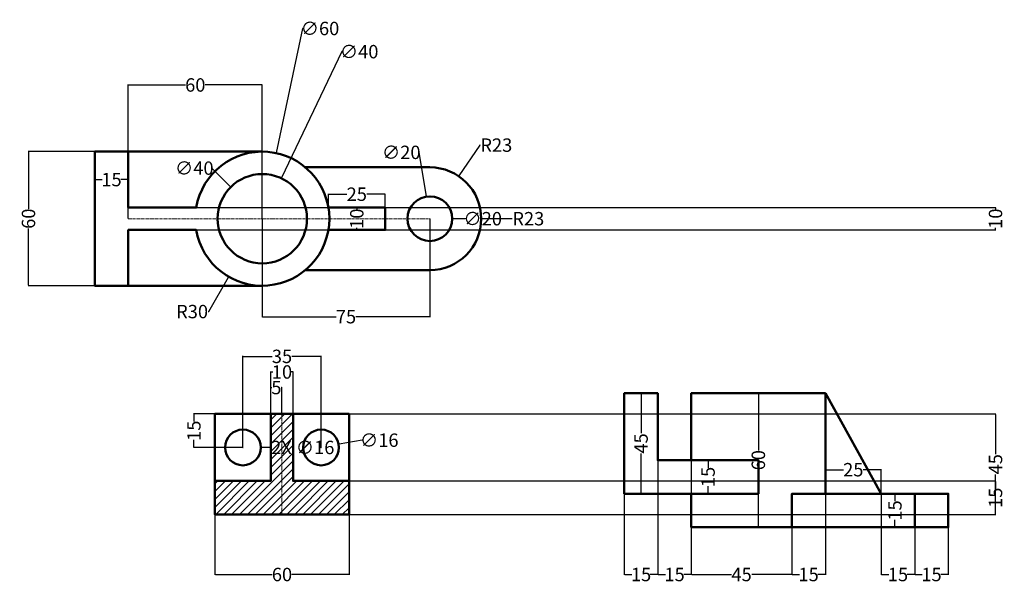
# Model space of a CAD drawing. Units: millimetres. Extents: x -22 to 419, y -106 to 146.
import ezdxf

# ---------------------------------------------------------------- set-up
doc = ezdxf.new("R2010")
doc.units = ezdxf.units.MM
doc.header["$MEASUREMENT"] = 0
doc.linetypes.add('CENTER', pattern=[2, 1.25, -0.25, 0.25, -0.25])
for name, color, linetype, lineweight in [('M-CNTR', 4, 'CENTER', 18), ('M-DIMS', 2, 'Continuous', 25), ('M-HATC', 8, 'Continuous', 18), ('M-OUTL', 7, 'Continuous', 50)]:
    doc.layers.add(name, color=color, linetype=linetype, lineweight=lineweight)
doc.styles.get("Standard").update_dxf_attribs({"font": 'arial.ttf'})
doc.dimstyles.get("Standard").update_dxf_attribs({"dimtxt": 6, "dimasz": 0.18, "dimexe": 0.18, "dimexo": 0.0625, "dimgap": 0.09, "dimtad": 0, "dimtoh": 1, "dimdec": 0, "dimzin": 0, "dimdsep": 46, "dimtxsty": 'Standard', "dimcen": 0.09, "dimadec": 0, "dimazin": 0, "dimtfac": 1, "dimtdec": 0, "dimtofl": 0, "dimtmove": 0, "dimatfit": 3, "dimfxl": 1, "dimtolj": 1, "dimtzin": 0, "dimarcsym": 0})

# ---------------------------------------------------------------- blocks, each defined once
blk = doc.blocks.new('*D1')
at = {"layer": 'Defpoints', "color": 0, "transparency": 16777216}
for p in [(12.03, 87.28), (-17.63, 27.28), (12.03, 27.28)]:
    blk.add_point(p, dxfattribs=at)
at = {"layer": 'M-DIMS', "color": 0, "lineweight": -2, "transparency": 16777216}
for p, q in [((11.96, 87.28), (-17.81, 87.28)), ((-17.63, 87.1), (-17.63, 61.67)), ((-17.63, 27.46), (-17.63, 52.89)), ((11.96, 27.28), (-17.81, 27.28))]:
    blk.add_line(p, q, dxfattribs=at)
at = {"layer": 'M-DIMS', "color": 0, "transparency": 16777216}
for points in [[(-17.66, 87.1), (-17.6, 87.1), (-17.63, 87.28)], [(-17.66, 27.46), (-17.6, 27.46), (-17.63, 27.28)]]:
    blk.add_solid(points, dxfattribs=at)
at = {"layer": 'M-DIMS', "color": 0, "transparency": 16777216, "insert": (-17.63, 57.28), "char_height": 6, "attachment_point": 5, "rotation": 90}
blk.add_mtext('\\A1;60', dxfattribs=at)
blk = doc.blocks.new('*D2')
at = {"layer": 'Defpoints', "color": 0, "transparency": 16777216}
for p in [(87.03, 117.12), (27.03, 57.28), (87.03, 57.28)]:
    blk.add_point(p, dxfattribs=at)
at = {"layer": 'M-DIMS', "color": 0, "lineweight": -2, "transparency": 16777216}
for p, q in [((27.03, 57.34), (27.03, 117.3)), ((27.21, 117.12), (52.63, 117.12)), ((86.85, 117.12), (61.42, 117.12)), ((87.03, 57.34), (87.03, 117.3))]:
    blk.add_line(p, q, dxfattribs=at)
at = {"layer": 'M-DIMS', "color": 0, "transparency": 16777216}
for points in [[(27.21, 117.15), (27.21, 117.09), (27.03, 117.12)], [(86.85, 117.15), (86.85, 117.09), (87.03, 117.12)]]:
    blk.add_solid(points, dxfattribs=at)
at = {"layer": 'M-DIMS', "color": 0, "transparency": 16777216, "insert": (57.03, 117.12), "char_height": 6, "attachment_point": 5}
blk.add_mtext('\\A1;60', dxfattribs=at)
blk = doc.blocks.new('*D3')
at = {"layer": 'Defpoints', "color": 0, "transparency": 16777216}
for p in [(95.61, 75.34), (78.44, 39.22)]:
    blk.add_point(p, dxfattribs=at)
at = {"layer": 'M-DIMS', "color": 0, "lineweight": -2, "transparency": 16777216}
for p, q in [((122.55, 132.03), (95.69, 75.51)), ((122.73, 132.03), (122.55, 132.03)), ((87.03, 57.19), (87.03, 57.37)), ((86.94, 57.28), (87.12, 57.28))]:
    blk.add_line(p, q, dxfattribs=at)
at = {"layer": 'M-DIMS', "color": 0, "transparency": 16777216}
blk.add_solid([(95.66, 75.52), (95.72, 75.49), (95.61, 75.34)], dxfattribs=at)
at = {"layer": 'M-DIMS', "color": 0, "transparency": 16777216, "insert": (130.37, 132.03), "char_height": 6, "attachment_point": 5}
blk.add_mtext('\\A1;∅40', dxfattribs=at)
blk = doc.blocks.new('*D4')
at = {"layer": 'Defpoints', "color": 0, "transparency": 16777216}
for p in [(93.24, 86.63), (80.82, 27.93)]:
    blk.add_point(p, dxfattribs=at)
at = {"layer": 'M-DIMS', "color": 0, "lineweight": -2, "transparency": 16777216}
for p, q in [((105.03, 142.4), (93.27, 86.81)), ((105.21, 142.4), (105.03, 142.4)), ((87.03, 57.19), (87.03, 57.37)), ((86.94, 57.28), (87.12, 57.28))]:
    blk.add_line(p, q, dxfattribs=at)
at = {"layer": 'M-DIMS', "color": 0, "transparency": 16777216}
blk.add_solid([(93.24, 86.81), (93.3, 86.8), (93.24, 86.63)], dxfattribs=at)
at = {"layer": 'M-DIMS', "color": 0, "transparency": 16777216, "insert": (112.85, 142.4), "char_height": 6, "attachment_point": 5}
blk.add_mtext('\\A1;∅60', dxfattribs=at)
blk = doc.blocks.new('*D5')
at = {"layer": 'Defpoints', "color": 0, "transparency": 16777216}
for p in [(86.94, 57.28), (162.03, 57.28), (162.03, 13.43)]:
    blk.add_point(p, dxfattribs=at)
at = {"layer": 'M-DIMS', "color": 0, "lineweight": -2, "transparency": 16777216}
for p, q in [((86.94, 57.22), (86.94, 13.25)), ((162.03, 57.22), (162.03, 13.25)), ((87.12, 13.43), (120.1, 13.43)), ((161.85, 13.43), (128.87, 13.43))]:
    blk.add_line(p, q, dxfattribs=at)
at = {"layer": 'M-DIMS', "color": 0, "transparency": 16777216}
for points in [[(87.12, 13.46), (87.12, 13.4), (86.94, 13.43)], [(161.85, 13.46), (161.85, 13.4), (162.03, 13.43)]]:
    blk.add_solid(points, dxfattribs=at)
at = {"layer": 'M-DIMS', "color": 0, "transparency": 16777216, "insert": (124.48, 13.43), "char_height": 6, "attachment_point": 5}
blk.add_mtext('\\A1;75', dxfattribs=at)
blk = doc.blocks.new('*D6')
at = {"layer": 'Defpoints', "color": 0, "transparency": 16777216}
for p in [(27.03, 74.78), (12.03, 57.28), (27.03, 57.28)]:
    blk.add_point(p, dxfattribs=at)
at = {"layer": 'M-DIMS', "color": 0, "lineweight": -2, "transparency": 16777216}
for p, q in [((12.03, 57.34), (12.03, 74.96)), ((27.03, 57.34), (27.03, 74.96)), ((12.21, 74.78), (15.4, 74.78)), ((26.85, 74.78), (23.65, 74.78))]:
    blk.add_line(p, q, dxfattribs=at)
at = {"layer": 'M-DIMS', "color": 0, "transparency": 16777216}
for points in [[(12.21, 74.81), (12.21, 74.75), (12.03, 74.78)], [(26.85, 74.81), (26.85, 74.75), (27.03, 74.78)]]:
    blk.add_solid(points, dxfattribs=at)
at = {"layer": 'M-DIMS', "color": 0, "transparency": 16777216, "insert": (19.53, 74.78), "char_height": 6, "attachment_point": 5}
blk.add_mtext('\\A1;15', dxfattribs=at)
blk = doc.blocks.new('*D7')
at = {"layer": 'Defpoints', "color": 0, "transparency": 16777216}
for p in [(129.32, 62.28), (129.32, 52.28), (129.32, 52.28)]:
    blk.add_point(p, dxfattribs=at)
at = {"layer": 'M-DIMS', "color": 0, "lineweight": -2, "transparency": 16777216}
for p, q in [((129.32, 62.1), (129.32, 61.38)), ((129.38, 62.28), (129.5, 62.28)), ((129.32, 52.46), (129.32, 53.19)), ((129.38, 52.28), (129.5, 52.28))]:
    blk.add_line(p, q, dxfattribs=at)
at = {"layer": 'M-DIMS', "color": 0, "transparency": 16777216}
for points in [[(129.29, 62.1), (129.35, 62.1), (129.32, 62.28)], [(129.29, 52.46), (129.35, 52.46), (129.32, 52.28)]]:
    blk.add_solid(points, dxfattribs=at)
at = {"layer": 'M-DIMS', "color": 0, "transparency": 16777216, "insert": (129.32, 57.28), "char_height": 6, "attachment_point": 5, "rotation": 90}
blk.add_mtext('\\A1;10', dxfattribs=at)
blk = doc.blocks.new('*D8')
at = {"layer": 'Defpoints', "color": 0, "transparency": 16777216}
for p in [(142.03, 68.24), (116.61, 62.28), (142.03, 62.28)]:
    blk.add_point(p, dxfattribs=at)
at = {"layer": 'M-DIMS', "color": 0, "lineweight": -2, "transparency": 16777216}
for p, q in [((116.61, 62.34), (116.61, 68.42)), ((116.79, 68.24), (124.86, 68.24)), ((141.85, 68.24), (133.78, 68.24)), ((142.03, 62.34), (142.03, 68.42))]:
    blk.add_line(p, q, dxfattribs=at)
at = {"layer": 'M-DIMS', "color": 0, "transparency": 16777216}
for points in [[(116.79, 68.27), (116.79, 68.21), (116.61, 68.24)], [(141.85, 68.27), (141.85, 68.21), (142.03, 68.24)]]:
    blk.add_solid(points, dxfattribs=at)
at = {"layer": 'M-DIMS', "color": 0, "transparency": 16777216, "insert": (129.32, 68.24), "char_height": 6, "attachment_point": 5}
blk.add_mtext('\\A1;25', dxfattribs=at)
blk = doc.blocks.new('*D9')
at = {"layer": 'Defpoints', "color": 0, "transparency": 16777216}
for p in [(174.92, 76.32), (162.03, 57.28)]:
    blk.add_point(p, dxfattribs=at)
at = {"layer": 'M-DIMS', "color": 0, "lineweight": -2, "transparency": 16777216}
for p, q in [((184.33, 90.21), (175.03, 76.47)), ((184.51, 90.21), (184.33, 90.21)), ((162.03, 57.19), (162.03, 57.37)), ((161.94, 57.28), (162.12, 57.28))]:
    blk.add_line(p, q, dxfattribs=at)
at = {"layer": 'M-DIMS', "color": 0, "transparency": 16777216}
blk.add_solid([(175, 76.49), (175.05, 76.46), (174.92, 76.32)], dxfattribs=at)
at = {"layer": 'M-DIMS', "color": 0, "transparency": 16777216, "insert": (191.77, 90.21), "char_height": 6, "attachment_point": 5}
blk.add_mtext('\\A1;R23', dxfattribs=at)
blk = doc.blocks.new('*D10')
at = {"layer": 'Defpoints', "color": 0, "transparency": 16777216}
for p in [(160.37, 67.14), (163.69, 47.42)]:
    blk.add_point(p, dxfattribs=at)
at = {"layer": 'M-DIMS', "color": 0, "lineweight": -2, "transparency": 16777216}
for p, q in [((156.85, 86.96), (157.03, 86.96)), ((157.03, 86.96), (160.34, 67.32)), ((162.03, 57.19), (162.03, 57.37)), ((161.94, 57.28), (162.12, 57.28))]:
    blk.add_line(p, q, dxfattribs=at)
at = {"layer": 'M-DIMS', "color": 0, "transparency": 16777216}
blk.add_solid([(160.37, 67.32), (160.31, 67.31), (160.37, 67.14)], dxfattribs=at)
at = {"layer": 'M-DIMS', "color": 0, "transparency": 16777216, "insert": (149.21, 86.96), "char_height": 6, "attachment_point": 5}
blk.add_mtext('\\A1;∅20', dxfattribs=at)
blk = doc.blocks.new('*D11')
at = {"layer": 'Defpoints', "color": 0, "transparency": 16777216}
for p in [(95.84, -18.29), (90.84, -30.1), (95.84, -29.98)]:
    blk.add_point(p, dxfattribs=at)
at = {"layer": 'M-DIMS', "color": 0, "lineweight": -2, "transparency": 16777216}
for p, q in [((90.84, -30.03), (90.84, -18.11)), ((91.02, -18.29), (91.26, -18.29)), ((95.66, -18.29), (95.42, -18.29)), ((95.84, -29.91), (95.84, -18.11))]:
    blk.add_line(p, q, dxfattribs=at)
at = {"layer": 'M-DIMS', "color": 0, "transparency": 16777216}
for points in [[(91.02, -18.26), (91.02, -18.32), (90.84, -18.29)], [(95.66, -18.26), (95.66, -18.32), (95.84, -18.29)]]:
    blk.add_solid(points, dxfattribs=at)
at = {"layer": 'M-DIMS', "color": 0, "transparency": 16777216, "insert": (93.34, -18.29), "char_height": 6, "attachment_point": 5}
blk.add_mtext('\\A1;5', dxfattribs=at)
blk = doc.blocks.new('*D12')
at = {"layer": 'Defpoints', "color": 0, "transparency": 16777216}
for p in [(100.84, -11.31), (90.84, -30.1), (100.84, -30.1)]:
    blk.add_point(p, dxfattribs=at)
at = {"layer": 'M-DIMS', "color": 0, "lineweight": -2, "transparency": 16777216}
for p, q in [((90.84, -30.03), (90.84, -11.13)), ((91.02, -11.31), (91.75, -11.31)), ((100.66, -11.31), (99.94, -11.31)), ((100.84, -30.03), (100.84, -11.13))]:
    blk.add_line(p, q, dxfattribs=at)
at = {"layer": 'M-DIMS', "color": 0, "transparency": 16777216}
for points in [[(91.02, -11.28), (91.02, -11.34), (90.84, -11.31)], [(100.66, -11.28), (100.66, -11.34), (100.84, -11.31)]]:
    blk.add_solid(points, dxfattribs=at)
at = {"layer": 'M-DIMS', "color": 0, "transparency": 16777216, "insert": (95.84, -11.31), "char_height": 6, "attachment_point": 5}
blk.add_mtext('\\A1;10', dxfattribs=at)
blk = doc.blocks.new('*D13')
at = {"layer": 'Defpoints', "color": 0, "transparency": 16777216}
for p in [(113.34, -4.33), (78.34, -45.1), (113.34, -45.1)]:
    blk.add_point(p, dxfattribs=at)
at = {"layer": 'M-DIMS', "color": 0, "lineweight": -2, "transparency": 16777216}
for p, q in [((78.34, -45.03), (78.34, -4.15)), ((78.52, -4.33), (91.43, -4.33)), ((113.16, -4.33), (100.25, -4.33)), ((113.34, -45.03), (113.34, -4.15))]:
    blk.add_line(p, q, dxfattribs=at)
at = {"layer": 'M-DIMS', "color": 0, "transparency": 16777216}
for points in [[(78.52, -4.3), (78.52, -4.36), (78.34, -4.33)], [(113.16, -4.3), (113.16, -4.36), (113.34, -4.33)]]:
    blk.add_solid(points, dxfattribs=at)
at = {"layer": 'M-DIMS', "color": 0, "transparency": 16777216, "insert": (95.84, -4.33), "char_height": 6, "attachment_point": 5}
blk.add_mtext('\\A1;35', dxfattribs=at)
blk = doc.blocks.new('*D14')
at = {"layer": 'Defpoints', "color": 0, "transparency": 16777216}
for p in [(78.34, -30.1), (56.41, -45.1), (78.34, -45.1)]:
    blk.add_point(p, dxfattribs=at)
at = {"layer": 'M-DIMS', "color": 0, "lineweight": -2, "transparency": 16777216}
for p, q in [((78.28, -30.1), (56.23, -30.1)), ((56.41, -30.28), (56.41, -33.47)), ((56.41, -44.92), (56.41, -41.72)), ((78.28, -45.1), (56.23, -45.1))]:
    blk.add_line(p, q, dxfattribs=at)
at = {"layer": 'M-DIMS', "color": 0, "transparency": 16777216}
for points in [[(56.38, -30.28), (56.44, -30.28), (56.41, -30.1)], [(56.38, -44.92), (56.44, -44.92), (56.41, -45.1)]]:
    blk.add_solid(points, dxfattribs=at)
at = {"layer": 'M-DIMS', "color": 0, "transparency": 16777216, "insert": (56.41, -37.6), "char_height": 6, "attachment_point": 5, "rotation": 90}
blk.add_mtext('\\A1;15', dxfattribs=at)
blk = doc.blocks.new('*D15')
at = {"layer": 'Defpoints', "color": 0, "transparency": 16777216}
for p in [(121.22, -43.7), (105.46, -46.49)]:
    blk.add_point(p, dxfattribs=at)
at = {"layer": 'M-DIMS', "color": 0, "lineweight": -2, "transparency": 16777216}
for p, q in [((131.72, -41.84), (121.39, -43.67)), ((113.25, -45.1), (113.43, -45.1)), ((113.34, -45.19), (113.34, -45.01))]:
    blk.add_line(p, q, dxfattribs=at)
at = {"layer": 'M-DIMS', "color": 0, "transparency": 16777216}
blk.add_solid([(121.39, -43.64), (121.4, -43.7), (121.22, -43.7)], dxfattribs=at)
at = {"layer": 'M-DIMS', "color": 0, "transparency": 16777216, "insert": (139.37, -41.84), "char_height": 6, "attachment_point": 5}
blk.add_mtext('\\A1;∅16', dxfattribs=at)
blk = doc.blocks.new('*D16')
at = {"layer": 'Defpoints', "color": 0, "transparency": 16777216}
for p in [(364.05, -55.04), (339.05, -65.8), (364.05, -65.8)]:
    blk.add_point(p, dxfattribs=at)
at = {"layer": 'M-DIMS', "color": 0, "lineweight": -2, "transparency": 16777216}
for p, q in [((339.05, -65.73), (339.05, -54.86)), ((339.23, -55.04), (347.09, -55.04)), ((363.87, -55.04), (356.01, -55.04)), ((364.05, -65.73), (364.05, -54.86))]:
    blk.add_line(p, q, dxfattribs=at)
at = {"layer": 'M-DIMS', "color": 0, "transparency": 16777216}
for points in [[(339.23, -55.01), (339.23, -55.07), (339.05, -55.04)], [(363.87, -55.01), (363.87, -55.07), (364.05, -55.04)]]:
    blk.add_solid(points, dxfattribs=at)
at = {"layer": 'M-DIMS', "color": 0, "transparency": 16777216, "insert": (351.55, -55.04), "char_height": 6, "attachment_point": 5}
blk.add_mtext('\\A1;25', dxfattribs=at)
blk = doc.blocks.new('*D17')
at = {"layer": 'Defpoints', "color": 0, "transparency": 16777216}
for p in [(370.18, -65.8), (370.18, -80.8), (370.18, -80.8)]:
    blk.add_point(p, dxfattribs=at)
at = {"layer": 'M-DIMS', "color": 0, "lineweight": -2, "transparency": 16777216}
for p, q in [((370.18, -65.98), (370.18, -69.17)), ((370.24, -65.8), (370.36, -65.8)), ((370.18, -80.62), (370.18, -77.42)), ((370.24, -80.8), (370.36, -80.8))]:
    blk.add_line(p, q, dxfattribs=at)
at = {"layer": 'M-DIMS', "color": 0, "transparency": 16777216}
for points in [[(370.15, -65.98), (370.21, -65.98), (370.18, -65.8)], [(370.15, -80.62), (370.21, -80.62), (370.18, -80.8)]]:
    blk.add_solid(points, dxfattribs=at)
at = {"layer": 'M-DIMS', "color": 0, "transparency": 16777216, "insert": (370.18, -73.3), "char_height": 6, "attachment_point": 5, "rotation": 90}
blk.add_mtext('\\A1;15', dxfattribs=at)
blk = doc.blocks.new('*D18')
at = {"layer": 'Defpoints', "color": 0, "transparency": 16777216}
for p in [(286.55, -50.8), (286.55, -65.8), (286.55, -65.8)]:
    blk.add_point(p, dxfattribs=at)
at = {"layer": 'M-DIMS', "color": 0, "lineweight": -2, "transparency": 16777216}
for p, q in [((286.55, -50.98), (286.55, -54.17)), ((286.62, -50.8), (286.73, -50.8)), ((286.55, -65.62), (286.55, -62.42)), ((286.62, -65.8), (286.73, -65.8))]:
    blk.add_line(p, q, dxfattribs=at)
at = {"layer": 'M-DIMS', "color": 0, "transparency": 16777216}
for points in [[(286.52, -50.98), (286.58, -50.98), (286.55, -50.8)], [(286.52, -65.62), (286.58, -65.62), (286.55, -65.8)]]:
    blk.add_solid(points, dxfattribs=at)
at = {"layer": 'M-DIMS', "color": 0, "transparency": 16777216, "insert": (286.55, -58.3), "char_height": 6, "attachment_point": 5, "rotation": 90}
blk.add_mtext('\\A1;15', dxfattribs=at)
blk = doc.blocks.new('*D19')
at = {"layer": 'Defpoints', "color": 0, "transparency": 16777216}
for p in [(256.55, -20.8), (256.55, -65.8), (256.55, -65.8)]:
    blk.add_point(p, dxfattribs=at)
at = {"layer": 'M-DIMS', "color": 0, "lineweight": -2, "transparency": 16777216}
for p, q in [((256.55, -20.98), (256.55, -38.77)), ((256.62, -20.8), (256.73, -20.8)), ((256.55, -65.62), (256.55, -47.83)), ((256.62, -65.8), (256.73, -65.8))]:
    blk.add_line(p, q, dxfattribs=at)
at = {"layer": 'M-DIMS', "color": 0, "transparency": 16777216}
for points in [[(256.52, -20.98), (256.58, -20.98), (256.55, -20.8)], [(256.52, -65.62), (256.58, -65.62), (256.55, -65.8)]]:
    blk.add_solid(points, dxfattribs=at)
at = {"layer": 'M-DIMS', "color": 0, "transparency": 16777216, "insert": (256.55, -43.3), "char_height": 6, "attachment_point": 5, "rotation": 90}
blk.add_mtext('\\A1;45', dxfattribs=at)
blk = doc.blocks.new('*D20')
at = {"layer": 'Defpoints', "color": 0, "transparency": 16777216}
for p in [(309.05, -20.8), (309.05, -80.8), (309.05, -80.8)]:
    blk.add_point(p, dxfattribs=at)
at = {"layer": 'M-DIMS', "color": 0, "lineweight": -2, "transparency": 16777216}
for p, q in [((309.05, -20.98), (309.05, -46.4)), ((309.12, -20.8), (309.23, -20.8)), ((309.05, -80.62), (309.05, -55.19)), ((309.12, -80.8), (309.23, -80.8))]:
    blk.add_line(p, q, dxfattribs=at)
at = {"layer": 'M-DIMS', "color": 0, "transparency": 16777216}
for points in [[(309.02, -20.98), (309.08, -20.98), (309.05, -20.8)], [(309.02, -80.62), (309.08, -80.62), (309.05, -80.8)]]:
    blk.add_solid(points, dxfattribs=at)
at = {"layer": 'M-DIMS', "color": 0, "transparency": 16777216, "insert": (309.05, -50.8), "char_height": 6, "attachment_point": 5, "rotation": 90}
blk.add_mtext('\\A1;60', dxfattribs=at)
blk = doc.blocks.new('*D21')
at = {"layer": 'Defpoints', "color": 0, "transparency": 16777216}
for p in [(65.84, -75.1), (125.84, -75.1), (125.84, -101.95)]:
    blk.add_point(p, dxfattribs=at)
at = {"layer": 'M-DIMS', "color": 0, "lineweight": -2, "transparency": 16777216}
for p, q in [((65.84, -75.16), (65.84, -102.13)), ((125.84, -75.16), (125.84, -102.13)), ((66.02, -101.95), (91.45, -101.95)), ((125.66, -101.95), (100.23, -101.95))]:
    blk.add_line(p, q, dxfattribs=at)
at = {"layer": 'M-DIMS', "color": 0, "transparency": 16777216}
for points in [[(66.02, -101.92), (66.02, -101.98), (65.84, -101.95)], [(125.66, -101.92), (125.66, -101.98), (125.84, -101.95)]]:
    blk.add_solid(points, dxfattribs=at)
at = {"layer": 'M-DIMS', "color": 0, "transparency": 16777216, "insert": (95.84, -101.95), "char_height": 6, "attachment_point": 5}
blk.add_mtext('\\A1;60', dxfattribs=at)
blk = doc.blocks.new('*D22')
at = {"layer": 'Defpoints', "color": 0, "transparency": 16777216}
for p in [(125.84, -60.1), (125.84, -75.1), (415.2, -75.1)]:
    blk.add_point(p, dxfattribs=at)
at = {"layer": 'M-DIMS', "color": 0, "lineweight": -2, "transparency": 16777216}
for p, q in [((125.9, -60.1), (415.38, -60.1)), ((415.2, -60.28), (415.2, -63.47)), ((415.2, -74.92), (415.2, -71.72)), ((125.9, -75.1), (415.38, -75.1))]:
    blk.add_line(p, q, dxfattribs=at)
at = {"layer": 'M-DIMS', "color": 0, "transparency": 16777216}
for points in [[(415.17, -60.28), (415.23, -60.28), (415.2, -60.1)], [(415.17, -74.92), (415.23, -74.92), (415.2, -75.1)]]:
    blk.add_solid(points, dxfattribs=at)
at = {"layer": 'M-DIMS', "color": 0, "transparency": 16777216, "insert": (415.2, -67.6), "char_height": 6, "attachment_point": 5, "rotation": 90}
blk.add_mtext('\\A1;15', dxfattribs=at)
blk = doc.blocks.new('*D23')
at = {"layer": 'Defpoints', "color": 0, "transparency": 16777216}
for p in [(125.84, -30.1), (125.84, -75.1), (415.2, -75.1)]:
    blk.add_point(p, dxfattribs=at)
at = {"layer": 'M-DIMS', "color": 0, "lineweight": -2, "transparency": 16777216}
for p, q in [((125.9, -30.1), (415.38, -30.1)), ((415.2, -30.28), (415.2, -48.06)), ((415.2, -74.92), (415.2, -57.13)), ((125.9, -75.1), (415.38, -75.1))]:
    blk.add_line(p, q, dxfattribs=at)
at = {"layer": 'M-DIMS', "color": 0, "transparency": 16777216}
for points in [[(415.17, -30.28), (415.23, -30.28), (415.2, -30.1)], [(415.17, -74.92), (415.23, -74.92), (415.2, -75.1)]]:
    blk.add_solid(points, dxfattribs=at)
at = {"layer": 'M-DIMS', "color": 0, "transparency": 16777216, "insert": (415.2, -52.6), "char_height": 6, "attachment_point": 5, "rotation": 90}
blk.add_mtext('\\A1;45', dxfattribs=at)
blk = doc.blocks.new('*D24')
at = {"layer": 'Defpoints', "color": 0, "transparency": 16777216}
for p in [(27.03, 62.28), (27.03, 52.28), (415.2, 52.28)]:
    blk.add_point(p, dxfattribs=at)
at = {"layer": 'M-DIMS', "color": 0, "lineweight": -2, "transparency": 16777216}
for p, q in [((27.09, 62.28), (415.38, 62.28)), ((415.2, 62.1), (415.2, 61.38)), ((415.2, 52.46), (415.2, 53.19)), ((27.09, 52.28), (415.38, 52.28))]:
    blk.add_line(p, q, dxfattribs=at)
at = {"layer": 'M-DIMS', "color": 0, "transparency": 16777216}
for points in [[(415.17, 62.1), (415.23, 62.1), (415.2, 62.28)], [(415.17, 52.46), (415.23, 52.46), (415.2, 52.28)]]:
    blk.add_solid(points, dxfattribs=at)
at = {"layer": 'M-DIMS', "color": 0, "transparency": 16777216, "insert": (415.2, 57.28), "char_height": 6, "attachment_point": 5, "rotation": 90}
blk.add_mtext('\\A1;10', dxfattribs=at)
blk = doc.blocks.new('*D25')
at = {"layer": 'Defpoints', "color": 0, "transparency": 16777216}
for p in [(264.05, -50.8), (249.05, -65.8), (264.05, -101.95)]:
    blk.add_point(p, dxfattribs=at)
at = {"layer": 'M-DIMS', "color": 0, "lineweight": -2, "transparency": 16777216}
for p, q in [((264.05, -50.86), (264.05, -102.13)), ((249.05, -65.86), (249.05, -102.13)), ((249.23, -101.95), (252.43, -101.95)), ((263.87, -101.95), (260.68, -101.95))]:
    blk.add_line(p, q, dxfattribs=at)
at = {"layer": 'M-DIMS', "color": 0, "transparency": 16777216}
for points in [[(249.23, -101.92), (249.23, -101.98), (249.05, -101.95)], [(263.87, -101.92), (263.87, -101.98), (264.05, -101.95)]]:
    blk.add_solid(points, dxfattribs=at)
at = {"layer": 'M-DIMS', "color": 0, "transparency": 16777216, "insert": (256.55, -101.95), "char_height": 6, "attachment_point": 5}
blk.add_mtext('\\A1;15', dxfattribs=at)
blk = doc.blocks.new('*D26')
at = {"layer": 'Defpoints', "color": 0, "transparency": 16777216}
for p in [(264.05, -50.8), (279.05, -50.8), (279.05, -101.95)]:
    blk.add_point(p, dxfattribs=at)
at = {"layer": 'M-DIMS', "color": 0, "lineweight": -2, "transparency": 16777216}
for p, q in [((264.05, -50.86), (264.05, -102.13)), ((279.05, -50.86), (279.05, -102.13)), ((264.23, -101.95), (267.43, -101.95)), ((278.87, -101.95), (275.68, -101.95))]:
    blk.add_line(p, q, dxfattribs=at)
at = {"layer": 'M-DIMS', "color": 0, "transparency": 16777216}
for points in [[(264.23, -101.92), (264.23, -101.98), (264.05, -101.95)], [(278.87, -101.92), (278.87, -101.98), (279.05, -101.95)]]:
    blk.add_solid(points, dxfattribs=at)
at = {"layer": 'M-DIMS', "color": 0, "transparency": 16777216, "insert": (271.55, -101.95), "char_height": 6, "attachment_point": 5}
blk.add_mtext('\\A1;15', dxfattribs=at)
blk = doc.blocks.new('*D27')
at = {"layer": 'Defpoints', "color": 0, "transparency": 16777216}
for p in [(279.05, -80.8), (324.05, -80.8), (324.05, -101.95)]:
    blk.add_point(p, dxfattribs=at)
at = {"layer": 'M-DIMS', "color": 0, "lineweight": -2, "transparency": 16777216}
for p, q in [((279.05, -80.86), (279.05, -102.13)), ((324.05, -80.86), (324.05, -102.13)), ((279.23, -101.95), (297.02, -101.95)), ((323.87, -101.95), (306.08, -101.95))]:
    blk.add_line(p, q, dxfattribs=at)
at = {"layer": 'M-DIMS', "color": 0, "transparency": 16777216}
for points in [[(279.23, -101.92), (279.23, -101.98), (279.05, -101.95)], [(323.87, -101.92), (323.87, -101.98), (324.05, -101.95)]]:
    blk.add_solid(points, dxfattribs=at)
at = {"layer": 'M-DIMS', "color": 0, "transparency": 16777216, "insert": (301.55, -101.95), "char_height": 6, "attachment_point": 5}
blk.add_mtext('\\A1;45', dxfattribs=at)
blk = doc.blocks.new('*D28')
at = {"layer": 'Defpoints', "color": 0, "transparency": 16777216}
for p in [(339.05, -65.8), (324.05, -80.8), (339.05, -101.95)]:
    blk.add_point(p, dxfattribs=at)
at = {"layer": 'M-DIMS', "color": 0, "lineweight": -2, "transparency": 16777216}
for p, q in [((339.05, -65.86), (339.05, -102.13)), ((324.05, -80.86), (324.05, -102.13)), ((324.23, -101.95), (327.43, -101.95)), ((338.87, -101.95), (335.68, -101.95))]:
    blk.add_line(p, q, dxfattribs=at)
at = {"layer": 'M-DIMS', "color": 0, "transparency": 16777216}
for points in [[(324.23, -101.92), (324.23, -101.98), (324.05, -101.95)], [(338.87, -101.92), (338.87, -101.98), (339.05, -101.95)]]:
    blk.add_solid(points, dxfattribs=at)
at = {"layer": 'M-DIMS', "color": 0, "transparency": 16777216, "insert": (331.55, -101.95), "char_height": 6, "attachment_point": 5}
blk.add_mtext('\\A1;15', dxfattribs=at)
blk = doc.blocks.new('*D29')
at = {"layer": 'Defpoints', "color": 0, "transparency": 16777216}
for p in [(364.05, -65.8), (379.05, -65.8), (379.05, -101.95)]:
    blk.add_point(p, dxfattribs=at)
at = {"layer": 'M-DIMS', "color": 0, "lineweight": -2, "transparency": 16777216}
for p, q in [((364.05, -65.86), (364.05, -102.13)), ((379.05, -65.86), (379.05, -102.13)), ((364.23, -101.95), (367.43, -101.95)), ((378.87, -101.95), (375.68, -101.95))]:
    blk.add_line(p, q, dxfattribs=at)
at = {"layer": 'M-DIMS', "color": 0, "transparency": 16777216}
for points in [[(364.23, -101.92), (364.23, -101.98), (364.05, -101.95)], [(378.87, -101.92), (378.87, -101.98), (379.05, -101.95)]]:
    blk.add_solid(points, dxfattribs=at)
at = {"layer": 'M-DIMS', "color": 0, "transparency": 16777216, "insert": (371.55, -101.95), "char_height": 6, "attachment_point": 5}
blk.add_mtext('\\A1;15', dxfattribs=at)
blk = doc.blocks.new('*D30')
at = {"layer": 'Defpoints', "color": 0, "transparency": 16777216}
for p in [(379.05, -80.8), (394.05, -80.8), (394.05, -101.95)]:
    blk.add_point(p, dxfattribs=at)
at = {"layer": 'M-DIMS', "color": 0, "lineweight": -2, "transparency": 16777216}
for p, q in [((379.05, -80.86), (379.05, -102.13)), ((394.05, -80.86), (394.05, -102.13)), ((379.23, -101.95), (382.43, -101.95)), ((393.87, -101.95), (390.68, -101.95))]:
    blk.add_line(p, q, dxfattribs=at)
at = {"layer": 'M-DIMS', "color": 0, "transparency": 16777216}
for points in [[(379.23, -101.92), (379.23, -101.98), (379.05, -101.95)], [(393.87, -101.92), (393.87, -101.98), (394.05, -101.95)]]:
    blk.add_solid(points, dxfattribs=at)
at = {"layer": 'M-DIMS', "color": 0, "transparency": 16777216, "insert": (386.55, -101.95), "char_height": 6, "attachment_point": 5}
blk.add_mtext('\\A1;15', dxfattribs=at)
blk = doc.blocks.new('*D31')
at = {"layer": 'Defpoints', "color": 0, "transparency": 16777216}
for p in [(87.03, 57.28), (72.03, 31.3)]:
    blk.add_point(p, dxfattribs=at)
at = {"layer": 'M-DIMS', "color": 0, "lineweight": -2, "transparency": 16777216}
for p, q in [((87.03, 57.19), (87.03, 57.37)), ((86.94, 57.28), (87.12, 57.28)), ((63.03, 15.71), (71.94, 31.14)), ((62.85, 15.71), (63.03, 15.71))]:
    blk.add_line(p, q, dxfattribs=at)
at = {"layer": 'M-DIMS', "color": 0, "transparency": 16777216}
blk.add_solid([(71.91, 31.16), (71.96, 31.13), (72.03, 31.3)], dxfattribs=at)
at = {"layer": 'M-DIMS', "color": 0, "transparency": 16777216, "insert": (55.6, 15.71), "char_height": 6, "attachment_point": 5}
blk.add_mtext('\\A1;R30', dxfattribs=at)
blk = doc.blocks.new('*D32')
at = {"layer": 'Defpoints', "color": 0, "transparency": 16777216}
for p in [(72.89, 71.42), (101.17, 43.14)]:
    blk.add_point(p, dxfattribs=at)
at = {"layer": 'M-DIMS', "color": 0, "lineweight": -2, "transparency": 16777216}
for p, q in [((64.22, 79.91), (64.4, 79.91)), ((64.4, 79.91), (72.76, 71.55)), ((87.03, 57.19), (87.03, 57.37)), ((86.94, 57.28), (87.12, 57.28))]:
    blk.add_line(p, q, dxfattribs=at)
at = {"layer": 'M-DIMS', "color": 0, "transparency": 16777216}
blk.add_solid([(72.78, 71.57), (72.74, 71.53), (72.89, 71.42)], dxfattribs=at)
at = {"layer": 'M-DIMS', "color": 0, "transparency": 16777216, "insert": (56.58, 79.91), "char_height": 6, "attachment_point": 5}
blk.add_mtext('\\A1;∅40', dxfattribs=at)
blk = doc.blocks.new('*D33')
at = {"layer": 'Defpoints', "color": 0, "transparency": 16777216}
for p in [(162.03, 57.28), (185.03, 57.28)]:
    blk.add_point(p, dxfattribs=at)
at = {"layer": 'M-DIMS', "color": 0, "lineweight": -2, "transparency": 16777216}
for p, q in [((162.03, 57.19), (162.03, 57.37)), ((161.94, 57.28), (162.12, 57.28)), ((198.83, 57.28), (185.21, 57.28))]:
    blk.add_line(p, q, dxfattribs=at)
at = {"layer": 'M-DIMS', "color": 0, "transparency": 16777216}
blk.add_solid([(185.21, 57.31), (185.21, 57.25), (185.03, 57.28)], dxfattribs=at)
at = {"layer": 'M-DIMS', "color": 0, "transparency": 16777216, "insert": (206.09, 57.28), "char_height": 6, "attachment_point": 5}
blk.add_mtext('\\A1;R23', dxfattribs=at)
blk = doc.blocks.new('*D34')
at = {"layer": 'Defpoints', "color": 0, "transparency": 16777216}
for p in [(152.03, 57.28), (172.03, 57.28)]:
    blk.add_point(p, dxfattribs=at)
at = {"layer": 'M-DIMS', "color": 0, "lineweight": -2, "transparency": 16777216}
for p, q in [((162.03, 57.19), (162.03, 57.37)), ((161.94, 57.28), (162.12, 57.28)), ((178.03, 57.28), (172.21, 57.28))]:
    blk.add_line(p, q, dxfattribs=at)
at = {"layer": 'M-DIMS', "color": 0, "transparency": 16777216}
blk.add_solid([(172.21, 57.31), (172.21, 57.25), (172.03, 57.28)], dxfattribs=at)
at = {"layer": 'M-DIMS', "color": 0, "transparency": 16777216, "insert": (185.67, 57.28), "char_height": 6, "attachment_point": 5}
blk.add_mtext('\\A1;∅20', dxfattribs=at)
blk = doc.blocks.new('*D35')
at = {"layer": 'Defpoints', "color": 0, "transparency": 16777216}
for p in [(70.34, -45.1), (86.34, -45.09)]:
    blk.add_point(p, dxfattribs=at)
at = {"layer": 'M-DIMS', "color": 0, "lineweight": -2, "transparency": 16777216}
for p, q in [((78.25, -45.1), (78.43, -45.1)), ((78.34, -45.19), (78.34, -45.01)), ((91.14, -45.09), (86.52, -45.09))]:
    blk.add_line(p, q, dxfattribs=at)
at = {"layer": 'M-DIMS', "color": 0, "transparency": 16777216}
blk.add_solid([(86.52, -45.06), (86.52, -45.12), (86.34, -45.09)], dxfattribs=at)
at = {"layer": 'M-DIMS', "color": 0, "transparency": 16777216, "insert": (105.13, -45.09), "char_height": 6, "attachment_point": 5}
blk.add_mtext('\\A1;2X ∅16', dxfattribs=at)

msp = doc.modelspace()

# ---------------------------------------------------------------- hatches: boundary and pattern name
at = {"layer": 'M-HATC'}
h = msp.add_hatch(dxfattribs=at)
h.set_pattern_fill('ANSI31', color=256, scale=20)
h.set_pattern_definition([(45, (0, 88.4952), (-1.767767, 1.767767), [])])
h.paths.add_polyline_path([(95.84, -30.1), (90.84, -30.1), (90.84, -60.1), (65.84, -60.1), (65.84, -75.1), (95.84, -75.1)])
h.paths.add_polyline_path([(100.84, -30.1), (95.84, -30.1), (95.84, -75.1), (125.84, -75.1), (125.84, -60.1), (100.84, -60.1)])

# ---------------------------------------------------------------- linework, layer by layer
at = {"layer": 'M-CNTR'}
msp.add_line((95.84, -29.98), (95.84, -75.22), dxfattribs=at)
for points in [[(87.03, 77.28), (87.03, 57.28), (142.03, 57.28), (162.03, 57.28)], [(27.03, 57.28), (47.03, 57.28), (87.03, 57.28), (87.03, 37.28)]]:
    msp.add_lwpolyline(points, dxfattribs=at)
at = {"layer": 'M-OUTL'}
for points in [[(27.03, 27.28), (12.03, 27.28), (12.03, 87.28), (27.03, 87.28)], [(116.61, 62.28), (142.03, 62.28), (142.03, 52.28), (116.61, 52.28)], [(339.05, -65.8), (339.05, -20.8), (309.05, -20.8), (279.05, -20.8), (279.05, -50.8)], [(339.05, -45.8), (339.05, -20.8), (364.05, -65.8), (370.18, -65.8)], [(65.84, -75.1), (125.84, -75.1), (125.84, -30.1), (65.84, -30.1), (65.84, -75.1), (65.84, -60.1), (90.84, -60.1), (90.84, -30.1)], [(125.84, -60.1), (100.84, -60.1), (100.84, -30.1)], [(279.05, -65.8), (279.05, -80.8), (339.05, -80.8)], [(353.56, -65.8), (339.05, -65.8), (324.05, -65.8), (324.05, -80.8), (379.05, -80.8)], [(346.31, -65.8), (394.05, -65.8), (394.05, -80.8), (379.05, -80.8), (379.05, -65.8)]]:
    msp.add_lwpolyline(points, dxfattribs=at)
for points in [[(87.03, 27.28), (27.03, 27.28), (27.03, 52.28), (57.45, 52.28, 11.91608), (57.45, 62.28), (27.03, 62.28), (27.03, 87.28), (87.03, 87.28)], [(106.29, 80.28), (162.03, 80.28, -1), (162.03, 34.28), (106.29, 34.28)]]:
    msp.add_lwpolyline(points, format="xyb", dxfattribs=at)
msp.add_lwpolyline([(249.05, -65.8), (309.05, -65.8), (309.05, -50.8), (264.05, -50.8), (264.05, -20.8), (249.05, -20.8)], close=True, dxfattribs=at)
for centre, radius in [((87.03, 57.28), 20), ((162.03, 57.28), 10), ((78.34, -45.1), 8), ((113.34, -45.1), 8)]:
    msp.add_circle(centre, radius, dxfattribs=at)

# ---------------------------------------------------------------- dimensions: what is measured, and where the dimension line sits
at = {"layer": 'M-DIMS'}
for p1, p2, override, picture, middle in [((80.82, 27.93), (93.24, 86.63), {"dimclrd": 0, "dimclre": 0, "dimclrt": 0}, '*D4', (112.85, 142.4)), ((78.44, 39.22), (95.61, 75.34), {"dimclrd": 0, "dimclre": 0, "dimclrt": 0}, '*D3', (130.37, 132.03)), ((163.69, 47.42), (160.37, 67.14), {"dimclrd": 0, "dimclre": 0, "dimclrt": 0}, '*D10', (149.21, 86.96)), ((101.17, 43.14), (72.89, 71.42), {"dimdec": 0, "dimlfac": 1, "dimrnd": 0, "dimzin": 0, "dimdsep": 46, "dimlunit": 2}, '*D32', (56.58, 79.91)), ((152.03, 57.28), (172.03, 57.28), {"dimdec": 0, "dimlfac": 1, "dimrnd": 0, "dimzin": 0, "dimdsep": 46, "dimlunit": 2}, '*D34', (178.03, 57.28)), ((105.46, -46.49), (121.22, -43.7), {"dimclrd": 0, "dimclre": 0, "dimclrt": 0}, '*D15', (131.72, -41.84))]:
    dim = msp.add_diameter_dim_2p(p1=p1, p2=p2, dimstyle='Standard', override=override, dxfattribs=at)
    dim.commit()
    dim.dimension.update_dxf_attribs({"geometry": picture, "text_midpoint": middle, "dimtype": 163})
for base, p1, p2, override, picture, middle in [((87.03, 117.12), (27.03, 57.28), (87.03, 57.28), {"dimclrd": 0, "dimclre": 0, "dimclrt": 0}, '*D2', (57.03, 117.12)), ((27.03, 74.78), (12.03, 57.28), (27.03, 57.28), {"dimclrd": 0, "dimclre": 0, "dimclrt": 0}, '*D6', (19.53, 74.78)), ((142.03, 68.24), (116.61, 62.28), (142.03, 62.28), {"dimclrd": 0, "dimclre": 0, "dimclrt": 0}, '*D8', (129.32, 68.24)), ((162.03, 13.43), (86.94, 57.28), (162.03, 57.28), {"dimclrd": 0, "dimclre": 0, "dimclrt": 0}, '*D5', (124.48, 13.43)), ((113.34, -4.33), (78.34, -45.1), (113.34, -45.1), {"dimclrd": 0, "dimclre": 0, "dimclrt": 0}, '*D13', (95.84, -4.33)), ((100.84, -11.31), (90.84, -30.1), (100.84, -30.1), {"dimclrd": 0, "dimclre": 0, "dimclrt": 0}, '*D12', (95.84, -11.31)), ((95.84, -18.29), (90.84, -30.1), (95.84, -29.98), {"dimclrd": 0, "dimclre": 0, "dimclrt": 0}, '*D11', (93.34, -18.29)), ((264.05, -101.95), (249.05, -65.8), (264.05, -50.8), {"dimdec": 0, "dimlfac": 1, "dimrnd": 0, "dimzin": 0, "dimdsep": 46, "dimlunit": 2}, '*D25', (256.55, -101.95)), ((279.05, -101.95), (264.05, -50.8), (279.05, -50.8), {"dimdec": 0, "dimlfac": 1, "dimrnd": 0, "dimzin": 0, "dimdsep": 46, "dimlunit": 2}, '*D26', (271.55, -101.95)), ((364.05, -55.04), (339.05, -65.8), (364.05, -65.8), {"dimclrd": 0, "dimclre": 0, "dimclrt": 0}, '*D16', (351.55, -55.04)), ((339.05, -101.95), (324.05, -80.8), (339.05, -65.8), {"dimdec": 0, "dimlfac": 1, "dimrnd": 0, "dimzin": 0, "dimdsep": 46, "dimlunit": 2}, '*D28', (331.55, -101.95)), ((379.05, -101.95), (364.05, -65.8), (379.05, -65.8), {"dimdec": 0, "dimlfac": 1, "dimrnd": 0, "dimzin": 0, "dimdsep": 46, "dimlunit": 2}, '*D29', (371.55, -101.95)), ((125.84, -101.95), (65.84, -75.1), (125.84, -75.1), {"dimdec": 0, "dimlfac": 1, "dimrnd": 0, "dimzin": 0, "dimdsep": 46, "dimlunit": 2}, '*D21', (95.84, -101.95)), ((324.05, -101.95), (279.05, -80.8), (324.05, -80.8), {"dimdec": 0, "dimlfac": 1, "dimrnd": 0, "dimzin": 0, "dimdsep": 46, "dimlunit": 2}, '*D27', (301.55, -101.95)), ((394.05, -101.95), (379.05, -80.8), (394.05, -80.8), {"dimdec": 0, "dimlfac": 1, "dimrnd": 0, "dimzin": 0, "dimdsep": 46, "dimlunit": 2}, '*D30', (386.55, -101.95))]:
    dim = msp.add_linear_dim(base=base, p1=p1, p2=p2, dimstyle='Standard', override=override, dxfattribs=at)
    dim.commit()
    dim.dimension.update_dxf_attribs({"geometry": picture, "text_midpoint": middle})
for center, mpoint, override, picture, middle in [((162.03, 57.28), (174.92, 76.32), {"dimclrd": 0, "dimclre": 0, "dimclrt": 0}, '*D9', (191.77, 90.21)), ((87.03, 57.28), (72.03, 31.3), {"dimdec": 0, "dimlfac": 1, "dimrnd": 0, "dimzin": 0, "dimdsep": 46, "dimlunit": 2}, '*D31', (55.6, 15.71)), ((162.03, 57.28), (185.03, 57.28), {"dimdec": 0, "dimlfac": 1, "dimrnd": 0, "dimzin": 0, "dimdsep": 46, "dimlunit": 2}, '*D33', (198.83, 57.28))]:
    dim = msp.add_radius_dim(center=center, mpoint=mpoint, dimstyle='Standard', override=override, dxfattribs=at)
    dim.commit()
    dim.dimension.update_dxf_attribs({"geometry": picture, "text_midpoint": middle, "dimtype": 164})
for base, p1, p2, override, picture, middle in [((-17.63, 27.28), (12.03, 87.28), (12.03, 27.28), {"dimclrd": 0, "dimclre": 0, "dimclrt": 0}, '*D1', (-17.63, 57.28)), ((415.2, 52.28), (27.03, 62.28), (27.03, 52.28), {"dimdec": 0, "dimlfac": 1, "dimrnd": 0, "dimzin": 0, "dimdsep": 46, "dimlunit": 2}, '*D24', (415.2, 57.28)), ((129.32, 52.28), (129.32, 62.28), (129.32, 52.28), {"dimclrd": 0, "dimclre": 0, "dimclrt": 0}, '*D7', (129.32, 57.28)), ((256.55, -65.8), (256.55, -20.8), (256.55, -65.8), {"dimclrd": 0, "dimclre": 0, "dimclrt": 0}, '*D19', (256.55, -43.3)), ((309.05, -80.8), (309.05, -20.8), (309.05, -80.8), {"dimclrd": 0, "dimclre": 0, "dimclrt": 0}, '*D20', (309.05, -50.8)), ((56.41, -45.1), (78.34, -30.1), (78.34, -45.1), {"dimclrd": 0, "dimclre": 0, "dimclrt": 0}, '*D14', (56.41, -37.6)), ((415.2, -75.1), (125.84, -30.1), (125.84, -75.1), {"dimdec": 0, "dimlfac": 1, "dimrnd": 0, "dimzin": 0, "dimdsep": 46, "dimlunit": 2}, '*D23', (415.2, -52.6)), ((286.55, -65.8), (286.55, -50.8), (286.55, -65.8), {"dimclrd": 0, "dimclre": 0, "dimclrt": 0}, '*D18', (286.55, -58.3)), ((415.2, -75.1), (125.84, -60.1), (125.84, -75.1), {"dimdec": 0, "dimlfac": 1, "dimrnd": 0, "dimzin": 0, "dimdsep": 46, "dimlunit": 2}, '*D22', (415.2, -67.6)), ((370.18, -80.8), (370.18, -65.8), (370.18, -80.8), {"dimclrd": 0, "dimclre": 0, "dimclrt": 0}, '*D17', (370.18, -73.3))]:
    dim = msp.add_linear_dim(base=base, p1=p1, p2=p2, angle=90, dimstyle='Standard', override=override, dxfattribs=at)
    dim.commit()
    dim.dimension.update_dxf_attribs({"geometry": picture, "text_midpoint": middle})
dim = msp.add_diameter_dim_2p(p1=(70.34, -45.1), p2=(86.34, -45.09), text='2X <>', dimstyle='Standard', override={"dimdec": 0, "dimlfac": 1, "dimrnd": 0, "dimzin": 0, "dimdsep": 46, "dimlunit": 2}, dxfattribs=at)
dim.commit()
dim.dimension.update_dxf_attribs({"geometry": '*D35', "text_midpoint": (91.14, -45.09), "dimtype": 163})

doc.saveas('drawing.dxf')
